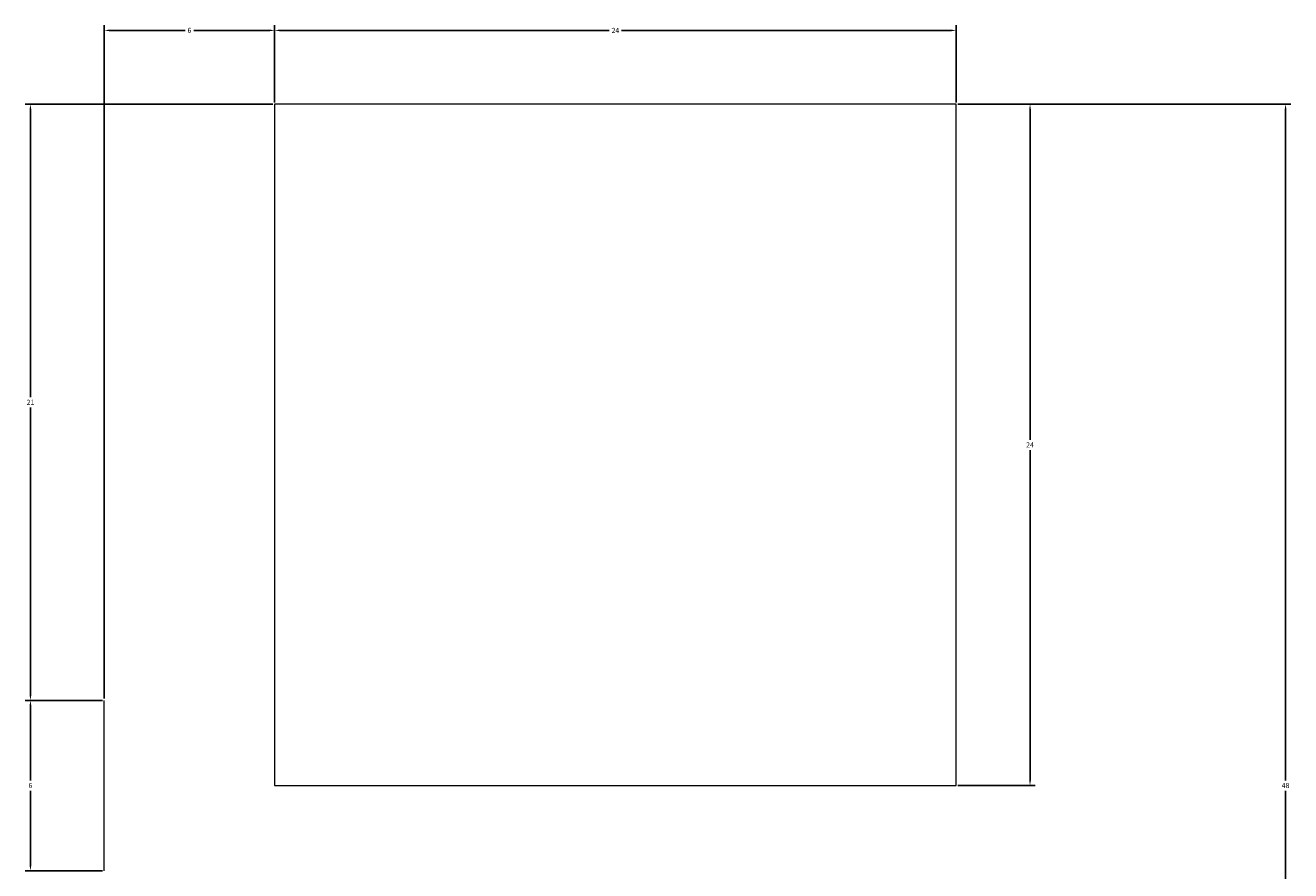
# Model space of a CAD drawing. Units: millimetres. Extents: x 3.7 to 48.2, y -50.7 to 2.9.
# Tile 2 of 2: x 3.7 to 48.2, y -26.9 to 2.9. Entities that reach past the tile are written whole.
import ezdxf

# ---------------------------------------------------------------- set-up
doc = ezdxf.new("R2010")
doc.units = ezdxf.units.MM
doc.header["$MEASUREMENT"] = 0
doc.layers.add('M-CONS', color=8, linetype='Continuous', lineweight=18)
doc.layers.add('M-DIMS', color=2, linetype='Continuous', lineweight=18)
doc.styles.get("Standard").update_dxf_attribs({"font": 'arial.ttf'})
doc.dimstyles.get("Standard").update_dxf_attribs({"dimtxt": 0.18, "dimasz": 0.18, "dimexe": 0.18, "dimexo": 0.0625, "dimgap": 0.09, "dimtad": 0, "dimtih": 1, "dimtoh": 1, "dimdec": 4, "dimzin": 0, "dimdsep": 46, "dimtxsty": 'Standard', "dimcen": 0.09, "dimadec": 0, "dimazin": 0, "dimtfac": 1, "dimtdec": 4, "dimtofl": 0, "dimtmove": 0, "dimatfit": 3, "dimfxl": 1, "dimtolj": 1, "dimtzin": 0, "dimarcsym": 0})

# ---------------------------------------------------------------- blocks, each defined once
blk = doc.blocks.new('*D1')
at = {"layer": 'Defpoints', "color": 0, "transparency": 16777216}
for p in [(36.456, 2.694), (12.456, 0.094), (36.456, 0.094)]:
    blk.add_point(p, dxfattribs=at)
at = {"layer": 'M-DIMS', "color": 0, "lineweight": -2, "transparency": 16777216}
for p, q in [((12.456, 0.156), (12.456, 2.874)), ((12.636, 2.694), (24.236, 2.694)), ((36.276, 2.694), (24.676, 2.694)), ((36.456, 0.156), (36.456, 2.874))]:
    blk.add_line(p, q, dxfattribs=at)
at = {"layer": 'M-DIMS', "color": 0, "transparency": 16777216}
for points in [[(12.636, 2.724), (12.636, 2.664), (12.456, 2.694)], [(36.276, 2.724), (36.276, 2.664), (36.456, 2.694)]]:
    blk.add_solid(points, dxfattribs=at)
at = {"layer": 'M-DIMS', "color": 0, "transparency": 16777216, "insert": (24.456, 2.694), "char_height": 0.18, "attachment_point": 5}
blk.add_mtext('\\A1;24', dxfattribs=at)
blk = doc.blocks.new('*D2')
at = {"layer": 'Defpoints', "color": 0, "transparency": 16777216}
for p in [(36.456, 0.094), (36.456, -23.906), (39.056, -23.906)]:
    blk.add_point(p, dxfattribs=at)
at = {"layer": 'M-DIMS', "color": 0, "lineweight": -2, "transparency": 16777216}
for p, q in [((36.518, 0.094), (39.236, 0.094)), ((39.056, -0.086), (39.056, -11.726)), ((39.056, -23.726), (39.056, -12.087)), ((36.518, -23.906), (39.236, -23.906))]:
    blk.add_line(p, q, dxfattribs=at)
at = {"layer": 'M-DIMS', "color": 0, "transparency": 16777216}
for points in [[(39.026, -0.086), (39.086, -0.086), (39.056, 0.094)], [(39.026, -23.726), (39.086, -23.726), (39.056, -23.906)]]:
    blk.add_solid(points, dxfattribs=at)
at = {"layer": 'M-DIMS', "color": 0, "transparency": 16777216, "insert": (39.056, -11.906), "char_height": 0.18, "attachment_point": 5}
blk.add_mtext('\\A1;24', dxfattribs=at)
blk = doc.blocks.new('*D4')
at = {"layer": 'Defpoints', "color": 0, "transparency": 16777216}
for p in [(36.456, 0.094), (45.456, -47.906), (48.056, -47.906)]:
    blk.add_point(p, dxfattribs=at)
at = {"layer": 'M-DIMS', "color": 0, "lineweight": -2, "transparency": 16777216}
for p, q in [((36.518, 0.094), (48.236, 0.094)), ((48.056, -0.086), (48.056, -23.724)), ((48.056, -47.726), (48.056, -24.088)), ((45.518, -47.906), (48.236, -47.906))]:
    blk.add_line(p, q, dxfattribs=at)
at = {"layer": 'M-DIMS', "color": 0, "transparency": 16777216}
for points in [[(48.026, -0.086), (48.086, -0.086), (48.056, 0.094)], [(48.026, -47.726), (48.086, -47.726), (48.056, -47.906)]]:
    blk.add_solid(points, dxfattribs=at)
at = {"layer": 'M-DIMS', "color": 0, "transparency": 16777216, "insert": (48.056, -23.906), "char_height": 0.18, "attachment_point": 5}
blk.add_mtext('\\A1;48', dxfattribs=at)
blk = doc.blocks.new('*D5')
at = {"layer": 'Defpoints', "color": 0, "transparency": 16777216}
for p in [(12.456, 2.694), (12.456, 0.094), (6.456, -20.906)]:
    blk.add_point(p, dxfattribs=at)
at = {"layer": 'M-DIMS', "color": 0, "lineweight": -2, "transparency": 16777216}
for p, q in [((6.456, -20.844), (6.456, 2.874)), ((6.636, 2.694), (9.306, 2.694)), ((12.276, 2.694), (9.605, 2.694)), ((12.456, 0.156), (12.456, 2.874))]:
    blk.add_line(p, q, dxfattribs=at)
at = {"layer": 'M-DIMS', "color": 0, "transparency": 16777216}
for points in [[(6.636, 2.724), (6.636, 2.664), (6.456, 2.694)], [(12.276, 2.724), (12.276, 2.664), (12.456, 2.694)]]:
    blk.add_solid(points, dxfattribs=at)
at = {"layer": 'M-DIMS', "color": 0, "transparency": 16777216, "insert": (9.456, 2.694), "char_height": 0.18, "attachment_point": 5}
blk.add_mtext('\\A1;6', dxfattribs=at)
blk = doc.blocks.new('*D6')
at = {"layer": 'Defpoints', "color": 0, "transparency": 16777216}
for p in [(3.856, -20.906), (6.456, -20.906), (6.456, -26.906)]:
    blk.add_point(p, dxfattribs=at)
at = {"layer": 'M-DIMS', "color": 0, "lineweight": -2, "transparency": 16777216}
for p, q in [((6.393, -20.906), (3.676, -20.906)), ((3.856, -21.086), (3.856, -23.724)), ((3.856, -26.726), (3.856, -24.088)), ((6.393, -26.906), (3.676, -26.906))]:
    blk.add_line(p, q, dxfattribs=at)
at = {"layer": 'M-DIMS', "color": 0, "transparency": 16777216}
for points in [[(3.826, -21.086), (3.886, -21.086), (3.856, -20.906)], [(3.826, -26.726), (3.886, -26.726), (3.856, -26.906)]]:
    blk.add_solid(points, dxfattribs=at)
at = {"layer": 'M-DIMS', "color": 0, "transparency": 16777216, "insert": (3.856, -23.906), "char_height": 0.18, "attachment_point": 5}
blk.add_mtext('\\A1;6', dxfattribs=at)
blk = doc.blocks.new('*D7')
at = {"layer": 'Defpoints', "color": 0, "transparency": 16777216}
for p in [(3.856, 0.094), (12.456, 0.094), (6.456, -20.906)]:
    blk.add_point(p, dxfattribs=at)
at = {"layer": 'M-DIMS', "color": 0, "lineweight": -2, "transparency": 16777216}
for p, q in [((12.393, 0.094), (3.676, 0.094)), ((3.856, -0.086), (3.856, -10.226)), ((3.856, -20.726), (3.856, -10.587)), ((6.393, -20.906), (3.676, -20.906))]:
    blk.add_line(p, q, dxfattribs=at)
at = {"layer": 'M-DIMS', "color": 0, "transparency": 16777216}
for points in [[(3.826, -0.086), (3.886, -0.086), (3.856, 0.094)], [(3.826, -20.726), (3.886, -20.726), (3.856, -20.906)]]:
    blk.add_solid(points, dxfattribs=at)
at = {"layer": 'M-DIMS', "color": 0, "transparency": 16777216, "insert": (3.856, -10.406), "char_height": 0.18, "attachment_point": 5}
blk.add_mtext('\\A1;21', dxfattribs=at)

msp = doc.modelspace()

# ---------------------------------------------------------------- linework, layer by layer
at = {"layer": 'M-CONS', "extrusion": (-1, -5e-16, 0)}
msp.add_line((6.456, -26.906, 27), (6.456, -20.906, 27), dxfattribs=at)
at = {"layer": 'M-CONS'}
msp.add_polyline3d([(36.456, -23.906, 27), (36.456, 0.094, 27), (12.456, 0.094, 27), (12.456, -23.906, 27)], close=True, dxfattribs=at)

# ---------------------------------------------------------------- dimensions: what is measured, and where the dimension line sits
at = {"layer": 'M-DIMS'}
for base, p1, p2, picture, middle in [((12.456, 2.694), (6.456, -20.906), (12.456, 0.094), '*D5', (9.456, 2.694)), ((36.456, 2.694), (12.456, 0.094), (36.456, 0.094), '*D1', (24.456, 2.694))]:
    dim = msp.add_linear_dim(base=base, p1=p1, p2=p2, dimstyle='Standard', override={"dimdec": 0, "dimlfac": 1, "dimrnd": 0, "dimzin": 0, "dimdsep": 46, "dimlunit": 2}, dxfattribs=at)
    dim.commit()
    dim.dimension.update_dxf_attribs({"geometry": picture, "text_midpoint": middle})
for base, p1, p2, angle, picture, middle in [((3.856, 0.094), (6.456, -20.906), (12.456, 0.094), 90, '*D7', (3.856, -10.406)), ((39.056, -23.906), (36.456, 0.094), (36.456, -23.906), 270, '*D2', (39.056, -11.906)), ((48.056, -47.906), (36.456, 0.094), (45.456, -47.906), 90, '*D4', (48.056, -23.906)), ((3.856, -20.906), (6.456, -26.906), (6.456, -20.906), 90, '*D6', (3.856, -23.906))]:
    dim = msp.add_linear_dim(base=base, p1=p1, p2=p2, angle=angle, dimstyle='Standard', override={"dimdec": 0, "dimlfac": 1, "dimrnd": 0, "dimzin": 0, "dimdsep": 46, "dimlunit": 2}, dxfattribs=at)
    dim.commit()
    dim.dimension.update_dxf_attribs({"geometry": picture, "text_midpoint": middle})

doc.saveas('drawing.dxf')
